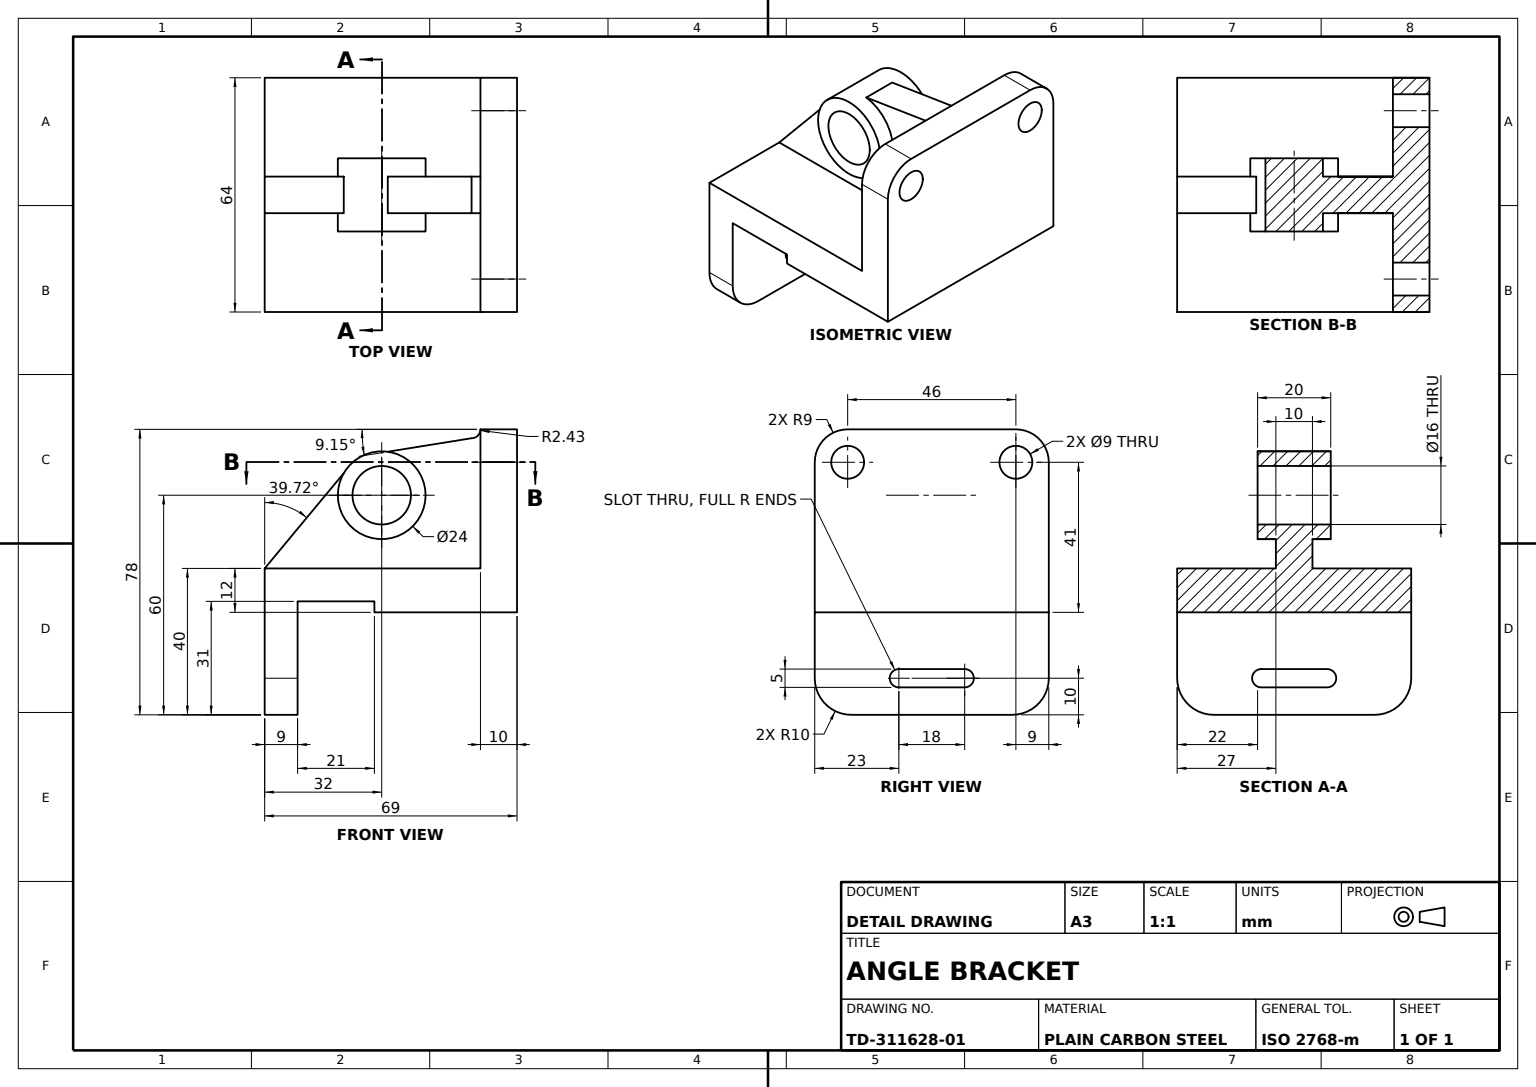
from build123d import *

# Parameters (mm, degrees)
BACK_PLATE_DEPTH        = 10
MOUNTING_HOLES_SKETCH_R = 4.5
MOUNTING_HOLES_2X_DEPTH = 10
L_BASE_BODY_DEPTH       = 64
HUB_BOSS_SKETCH_R       = 12
HUB_BOSS_DEPTH          = 10
SUPPORT_RIB_DEPTH       = 5
HUB_BORE_SKETCH_R       = 8
HUB_BORE_16_DEPTH       = 30
FRONT_SLOT_DEPTH        = 30
EDGE_FILLET_R10_A_R     = 10
EDGE_FILLET_R10_B_R     = 10


with BuildPart() as part:
    # Back Plate Sketch → Back Plate (new body)
    with BuildSketch(Plane.XY):
        with BuildLine():
            Line((0, 0), (0, 41))
            ThreePointArc((0, 41), (2.636038969, 47.363961031), (9, 50))
            Line((9, 50), (55, 50))
            ThreePointArc((55, 50), (61.363961031, 47.363961031), (64, 41))
            Line((64, 41), (64, 0))
            Line((64, 0), (0, 0))
        make_face()
    extrude(amount=BACK_PLATE_DEPTH)

    # Mounting Holes Sketch → Mounting Holes 2x (cut)
    with BuildSketch(Plane.XY.offset(10)):
        with Locations((9, 41)):
            Circle(MOUNTING_HOLES_SKETCH_R)
        with Locations((55, 41)):
            Circle(MOUNTING_HOLES_SKETCH_R)
    extrude(amount=-MOUNTING_HOLES_2X_DEPTH, mode=Mode.SUBTRACT)

    # L-Base Profile Sketch → L-Base Body (add)
    with BuildSketch(Plane.ZY):
        Polygon((0, 0), (39, 0), (39, 3), (60, 3), (60, -28), (69, -28), (69, 12), (0, 12), align=None)
    extrude(amount=-L_BASE_BODY_DEPTH)



with BuildPart() as body_2:
    # Hub Boss Sketch → Hub Boss (new, symmetric)
    with BuildSketch(Plane.ZY.offset(-32)):
        with Locations((37, 32)):
            Circle(HUB_BOSS_SKETCH_R)
    extrude(amount=HUB_BOSS_DEPTH, both=True)


with BuildPart() as part_1:
    add(part.part)

    add(body_2.part)  # Support Rib merges body 2
    # Support Rib Sketch → Support Rib (add, symmetric)
    with BuildSketch(Plane.ZY.offset(-32)):
        with BuildLine():
            Line((10, 12), (69, 12))
            Line((69, 12), (44.830635443, 41.092917494))
            Line((44.830635443, 41.092917494), (35.339623776, 43.884576172))
            Line((35.339623776, 43.884576172), (12.426606273, 47.573393727))
            ThreePointArc((12.426606273, 47.573393727), (10.710736522, 48.284130249), (10, 50))
            Line((10, 50), (10, 12))
        make_face()
    extrude(amount=SUPPORT_RIB_DEPTH, both=True)

    # Hub Bore Sketch → Hub Bore Ø16 (cut, symmetric)
    with BuildSketch(Plane.ZY.offset(-22)):
        with Locations((37, 32)):
            Circle(HUB_BORE_SKETCH_R)
    extrude(amount=HUB_BORE_16_DEPTH, both=True, mode=Mode.SUBTRACT)

    # Front Slot Sketch → Front Slot (cut, symmetric)
    with BuildSketch(Plane.XY.offset(69)):
        with BuildLine():
            Line((23, -15.5), (41, -15.5))
            ThreePointArc((41, -15.5), (43.5, -18), (41, -20.5))
            Line((41, -20.5), (23, -20.5))
            ThreePointArc((23, -20.5), (20.5, -18), (23, -15.5))
        make_face()
    extrude(amount=FRONT_SLOT_DEPTH, both=True, mode=Mode.SUBTRACT)

    # Edge Fillet R10 A
    edge_fillet_r10_a_edges = [part_1.edges().sort_by_distance(p)[0] for p in [
        (0, -28, 64.5),
    ]]
    fillet(edge_fillet_r10_a_edges, radius=EDGE_FILLET_R10_A_R)

    # Edge Fillet R10 B
    edge_fillet_r10_b_edges = [part_1.edges().sort_by_distance(p)[0] for p in [
        (64, -28, 64.5),
    ]]
    fillet(edge_fillet_r10_b_edges, radius=EDGE_FILLET_R10_B_R)


solid = part_1.part
